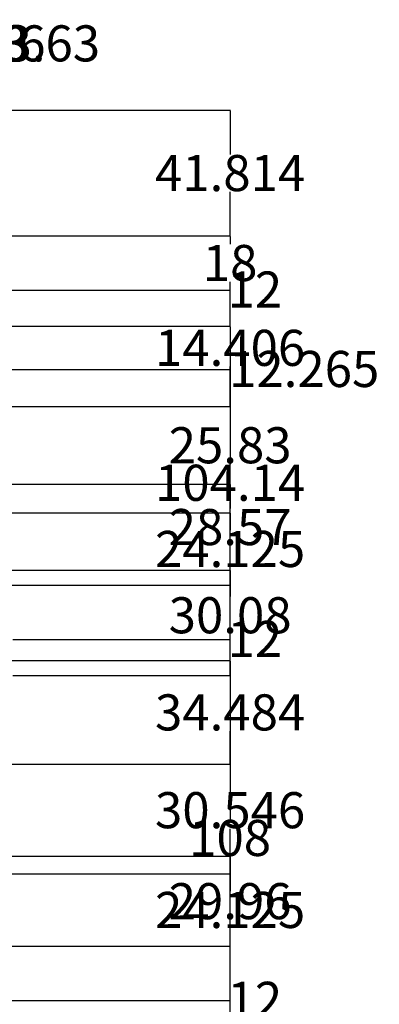
# Model space of a CAD drawing. Units: inches. Extents: x -73 to 458, y -161 to 332.
# Tile 6 of 6: x 338 to 458, y 5 to 332. Entities that reach past the tile are written whole.
import ezdxf

# ---------------------------------------------------------------- set-up
doc = ezdxf.new("R2010")
doc.units = ezdxf.units.IN
doc.header["$MEASUREMENT"] = 0
doc.layers.add('A-ANNO-DIMS', color=2, linetype='Continuous', lineweight=18)
doc.styles.get("Standard").update_dxf_attribs({"font": 'arial.ttf'})
doc.dimstyles.get("Standard").update_dxf_attribs({"dimtxt": 12, "dimasz": 0.18, "dimexe": 0.18, "dimexo": 0.0625, "dimgap": 0.09, "dimtad": 0, "dimtih": 1, "dimtoh": 1, "dimdec": 0, "dimzin": 0, "dimdsep": 46, "dimlunit": 3, "dimtxsty": 'Standard', "dimcen": 0.09, "dimadec": 0, "dimazin": 0, "dimtfac": 1, "dimtdec": 0, "dimtofl": 0, "dimtmove": 0, "dimatfit": 3, "dimfxl": 1, "dimtolj": 1, "dimtzin": 0, "dimarcsym": 0})

# ---------------------------------------------------------------- blocks, each defined once
blk = doc.blocks.new('*D18')
at = {"layer": 'A-ANNO-DIMS', "color": 0, "lineweight": -2, "transparency": 16777216}
for p, q in [((336.06, 6.07), (408.51, 6.07)), ((408.33, 6.07), (408.33, 6.25)), ((408.33, 6.25), (408.51, 6.25)), ((408.33, -5.75), (408.33, 5.89)), ((336.06, -5.93), (408.51, -5.93))]:
    blk.add_line(p, q, dxfattribs=at)
at = {"layer": 'A-ANNO-DIMS', "color": 0, "transparency": 16777216}
for points in [[(408.3, 5.89), (408.36, 5.89), (408.33, 6.07)], [(408.3, -5.75), (408.36, -5.75), (408.33, -5.93)]]:
    blk.add_solid(points, dxfattribs=at)
at = {"layer": 'Defpoints', "color": 0, "transparency": 16777216}
for p in [(336, 6.07), (408.33, 6.07), (336, -5.93)]:
    blk.add_point(p, dxfattribs=at)
at = {"layer": 'A-ANNO-DIMS', "color": 0, "transparency": 16777216, "insert": (416.56, 6.25), "char_height": 12, "attachment_point": 5}
blk.add_mtext('\\A1;12', dxfattribs=at)
blk = doc.blocks.new('*D20')
at = {"layer": 'A-ANNO-DIMS', "color": 0, "lineweight": -2, "transparency": 16777216}
for p, q in [((336.06, 114.07), (408.51, 114.07)), ((408.33, 113.89), (408.33, 66.28)), ((408.33, 6.25), (408.33, 53.85)), ((324.06, 6.07), (408.51, 6.07))]:
    blk.add_line(p, q, dxfattribs=at)
at = {"layer": 'A-ANNO-DIMS', "color": 0, "transparency": 16777216}
for points in [[(408.3, 113.89), (408.36, 113.89), (408.33, 114.07)], [(408.3, 6.25), (408.36, 6.25), (408.33, 6.07)]]:
    blk.add_solid(points, dxfattribs=at)
at = {"layer": 'Defpoints', "color": 0, "transparency": 16777216}
for p in [(336, 114.07), (408.33, 114.07), (324, 6.07)]:
    blk.add_point(p, dxfattribs=at)
at = {"layer": 'A-ANNO-DIMS', "color": 0, "transparency": 16777216, "insert": (408.33, 60.07), "char_height": 12, "attachment_point": 5}
blk.add_mtext('\\A1;108', dxfattribs=at)
blk = doc.blocks.new('*D21')
at = {"layer": 'A-ANNO-DIMS', "color": 0, "lineweight": -2, "transparency": 16777216}
for p, q in [((336.06, 126.07), (408.51, 126.07)), ((408.33, 126.07), (408.33, 126.25)), ((408.33, 126.25), (408.51, 126.25)), ((408.33, 114.25), (408.33, 125.89)), ((336.06, 114.07), (408.51, 114.07))]:
    blk.add_line(p, q, dxfattribs=at)
at = {"layer": 'A-ANNO-DIMS', "color": 0, "transparency": 16777216}
for points in [[(408.3, 125.89), (408.36, 125.89), (408.33, 126.07)], [(408.3, 114.25), (408.36, 114.25), (408.33, 114.07)]]:
    blk.add_solid(points, dxfattribs=at)
at = {"layer": 'Defpoints', "color": 0, "transparency": 16777216}
for p in [(336, 126.07), (408.33, 126.07), (336, 114.07)]:
    blk.add_point(p, dxfattribs=at)
at = {"layer": 'A-ANNO-DIMS', "color": 0, "transparency": 16777216, "insert": (416.56, 126.25), "char_height": 12, "attachment_point": 5}
blk.add_mtext('\\A1;12', dxfattribs=at)
blk = doc.blocks.new('*D22')
at = {"layer": 'A-ANNO-DIMS', "color": 0, "lineweight": -2, "transparency": 16777216}
for p, q in [((336.06, 230.21), (408.51, 230.21)), ((408.33, 230.03), (408.33, 184.35)), ((408.33, 126.25), (408.33, 171.92)), ((336.06, 126.07), (408.51, 126.07))]:
    blk.add_line(p, q, dxfattribs=at)
at = {"layer": 'A-ANNO-DIMS', "color": 0, "transparency": 16777216}
for points in [[(408.3, 230.03), (408.36, 230.03), (408.33, 230.21)], [(408.3, 126.25), (408.36, 126.25), (408.33, 126.07)]]:
    blk.add_solid(points, dxfattribs=at)
at = {"layer": 'Defpoints', "color": 0, "transparency": 16777216}
for p in [(336, 230.21), (408.33, 230.21), (336, 126.07)]:
    blk.add_point(p, dxfattribs=at)
at = {"layer": 'A-ANNO-DIMS', "color": 0, "transparency": 16777216, "insert": (408.33, 178.14), "char_height": 12, "attachment_point": 5}
blk.add_mtext('\\A1;104.14', dxfattribs=at)
blk = doc.blocks.new('*D23')
at = {"layer": 'A-ANNO-DIMS', "color": 0, "lineweight": -2, "transparency": 16777216}
for p, q in [((408.33, 242.21), (408.33, 242.39)), ((408.33, 242.39), (408.51, 242.39)), ((336.06, 242.21), (408.51, 242.21)), ((408.33, 230.39), (408.33, 242.03)), ((336.06, 230.21), (408.51, 230.21))]:
    blk.add_line(p, q, dxfattribs=at)
at = {"layer": 'A-ANNO-DIMS', "color": 0, "transparency": 16777216}
for points in [[(408.3, 242.03), (408.36, 242.03), (408.33, 242.21)], [(408.3, 230.39), (408.36, 230.39), (408.33, 230.21)]]:
    blk.add_solid(points, dxfattribs=at)
at = {"layer": 'Defpoints', "color": 0, "transparency": 16777216}
for p in [(336, 242.21), (408.33, 242.21), (336, 230.21)]:
    blk.add_point(p, dxfattribs=at)
at = {"layer": 'A-ANNO-DIMS', "color": 0, "transparency": 16777216, "insert": (416.56, 242.39), "char_height": 12, "attachment_point": 5}
blk.add_mtext('\\A1;12', dxfattribs=at)
blk = doc.blocks.new('*D24')
at = {"layer": 'A-ANNO-DIMS', "color": 0, "lineweight": -2, "transparency": 16777216}
for p, q in [((324.06, 260.21), (408.51, 260.21)), ((408.33, 260.03), (408.33, 257.42)), ((408.33, 242.39), (408.33, 244.99)), ((324.06, 242.21), (408.51, 242.21))]:
    blk.add_line(p, q, dxfattribs=at)
at = {"layer": 'A-ANNO-DIMS', "color": 0, "transparency": 16777216}
for points in [[(408.3, 260.03), (408.36, 260.03), (408.33, 260.21)], [(408.3, 242.39), (408.36, 242.39), (408.33, 242.21)]]:
    blk.add_solid(points, dxfattribs=at)
at = {"layer": 'Defpoints', "color": 0, "transparency": 16777216}
for p in [(324, 260.21), (408.33, 260.21), (324, 242.21)]:
    blk.add_point(p, dxfattribs=at)
at = {"layer": 'A-ANNO-DIMS', "color": 0, "transparency": 16777216, "insert": (408.33, 251.21), "char_height": 12, "attachment_point": 5}
blk.add_mtext('\\A1;18', dxfattribs=at)
blk = doc.blocks.new('*D25')
at = {"layer": 'A-ANNO-DIMS', "color": 0, "lineweight": -2, "transparency": 16777216}
for p, q in [((168.06, 302.02), (408.51, 302.02)), ((408.33, 301.84), (408.33, 287.33)), ((408.33, 260.39), (408.33, 274.9)), ((168.06, 260.21), (408.51, 260.21))]:
    blk.add_line(p, q, dxfattribs=at)
at = {"layer": 'A-ANNO-DIMS', "color": 0, "transparency": 16777216}
for points in [[(408.3, 301.84), (408.36, 301.84), (408.33, 302.02)], [(408.3, 260.39), (408.36, 260.39), (408.33, 260.21)]]:
    blk.add_solid(points, dxfattribs=at)
at = {"layer": 'Defpoints', "color": 0, "transparency": 16777216}
for p in [(168, 302.02), (408.33, 302.02), (168, 260.21)]:
    blk.add_point(p, dxfattribs=at)
at = {"layer": 'A-ANNO-DIMS', "color": 0, "transparency": 16777216, "insert": (408.33, 281.11), "char_height": 12, "attachment_point": 5}
blk.add_mtext('\\A1;41.814', dxfattribs=at)
blk = doc.blocks.new('*D39')
at = {"layer": 'A-ANNO-DIMS', "color": 0, "lineweight": -2, "transparency": 16777216}
for p, q in [((144.06, 54.03), (408.51, 54.03)), ((408.33, 53.85), (408.33, 45.26)), ((408.33, 24.25), (408.33, 32.83)), ((144.06, 24.07), (408.51, 24.07))]:
    blk.add_line(p, q, dxfattribs=at)
at = {"layer": 'A-ANNO-DIMS', "color": 0, "transparency": 16777216}
for points in [[(408.3, 53.85), (408.36, 53.85), (408.33, 54.03)], [(408.3, 24.25), (408.36, 24.25), (408.33, 24.07)]]:
    blk.add_solid(points, dxfattribs=at)
at = {"layer": 'Defpoints', "color": 0, "transparency": 16777216}
for p in [(144, 54.03), (408.33, 54.03), (144, 24.07)]:
    blk.add_point(p, dxfattribs=at)
at = {"layer": 'A-ANNO-DIMS', "color": 0, "transparency": 16777216, "insert": (408.33, 39.05), "char_height": 12, "attachment_point": 5}
blk.add_mtext('\\A1;29.96', dxfattribs=at)
blk = doc.blocks.new('*D40')
at = {"layer": 'A-ANNO-DIMS', "color": 0, "lineweight": -2, "transparency": 16777216}
for p, q in [((144.06, 84.57), (408.51, 84.57)), ((408.33, 84.39), (408.33, 75.52)), ((408.33, 54.21), (408.33, 63.08)), ((144.06, 54.03), (408.51, 54.03))]:
    blk.add_line(p, q, dxfattribs=at)
at = {"layer": 'A-ANNO-DIMS', "color": 0, "transparency": 16777216}
for points in [[(408.3, 84.39), (408.36, 84.39), (408.33, 84.57)], [(408.3, 54.21), (408.36, 54.21), (408.33, 54.03)]]:
    blk.add_solid(points, dxfattribs=at)
at = {"layer": 'Defpoints', "color": 0, "transparency": 16777216}
for p in [(144, 84.57), (408.33, 84.57), (144, 54.03)]:
    blk.add_point(p, dxfattribs=at)
at = {"layer": 'A-ANNO-DIMS', "color": 0, "transparency": 16777216, "insert": (408.33, 69.3), "char_height": 12, "attachment_point": 5}
blk.add_mtext('\\A1;30.546', dxfattribs=at)
blk = doc.blocks.new('*D41')
at = {"layer": 'A-ANNO-DIMS', "color": 0, "lineweight": -2, "transparency": 16777216}
for p, q in [((144.06, 119.06), (408.51, 119.06)), ((408.33, 118.88), (408.33, 108.04)), ((408.33, 84.75), (408.33, 95.59)), ((144.06, 84.57), (408.51, 84.57))]:
    blk.add_line(p, q, dxfattribs=at)
at = {"layer": 'A-ANNO-DIMS', "color": 0, "transparency": 16777216}
for points in [[(408.3, 118.88), (408.36, 118.88), (408.33, 119.06)], [(408.3, 84.75), (408.36, 84.75), (408.33, 84.57)]]:
    blk.add_solid(points, dxfattribs=at)
at = {"layer": 'Defpoints', "color": 0, "transparency": 16777216}
for p in [(144, 119.06), (408.33, 119.06), (144, 84.57)]:
    blk.add_point(p, dxfattribs=at)
at = {"layer": 'A-ANNO-DIMS', "color": 0, "transparency": 16777216, "insert": (408.33, 101.81), "char_height": 12, "attachment_point": 5}
blk.add_mtext('\\A1;34.484', dxfattribs=at)
blk = doc.blocks.new('*D42')
at = {"layer": 'A-ANNO-DIMS', "color": 0, "lineweight": -2, "transparency": 16777216}
for p, q in [((144.06, 149.14), (408.51, 149.14)), ((408.33, 148.96), (408.33, 140.32)), ((408.33, 119.24), (408.33, 127.88)), ((144.06, 119.06), (408.51, 119.06))]:
    blk.add_line(p, q, dxfattribs=at)
at = {"layer": 'A-ANNO-DIMS', "color": 0, "transparency": 16777216}
for points in [[(408.3, 148.96), (408.36, 148.96), (408.33, 149.14)], [(408.3, 119.24), (408.36, 119.24), (408.33, 119.06)]]:
    blk.add_solid(points, dxfattribs=at)
at = {"layer": 'Defpoints', "color": 0, "transparency": 16777216}
for p in [(144, 149.14), (408.33, 149.14), (144, 119.06)]:
    blk.add_point(p, dxfattribs=at)
at = {"layer": 'A-ANNO-DIMS', "color": 0, "transparency": 16777216, "insert": (408.33, 134.1), "char_height": 12, "attachment_point": 5}
blk.add_mtext('\\A1;30.08', dxfattribs=at)
blk = doc.blocks.new('*D43')
at = {"layer": 'A-ANNO-DIMS', "color": 0, "lineweight": -2, "transparency": 16777216}
for p, q in [((144.06, 177.7), (408.51, 177.7)), ((408.33, 177.52), (408.33, 169.64)), ((408.33, 149.32), (408.33, 157.2)), ((144.06, 149.14), (408.51, 149.14))]:
    blk.add_line(p, q, dxfattribs=at)
at = {"layer": 'A-ANNO-DIMS', "color": 0, "transparency": 16777216}
for points in [[(408.3, 177.52), (408.36, 177.52), (408.33, 177.7)], [(408.3, 149.32), (408.36, 149.32), (408.33, 149.14)]]:
    blk.add_solid(points, dxfattribs=at)
at = {"layer": 'Defpoints', "color": 0, "transparency": 16777216}
for p in [(144, 177.7), (408.33, 177.7), (144, 149.14)]:
    blk.add_point(p, dxfattribs=at)
at = {"layer": 'A-ANNO-DIMS', "color": 0, "transparency": 16777216, "insert": (408.33, 163.42), "char_height": 12, "attachment_point": 5}
blk.add_mtext('\\A1;28.57', dxfattribs=at)
blk = doc.blocks.new('*D44')
at = {"layer": 'A-ANNO-DIMS', "color": 0, "lineweight": -2, "transparency": 16777216}
for p, q in [((144.06, 203.54), (408.51, 203.54)), ((408.33, 203.36), (408.33, 196.84)), ((408.33, 177.88), (408.33, 184.4)), ((144.06, 177.7), (408.51, 177.7))]:
    blk.add_line(p, q, dxfattribs=at)
at = {"layer": 'A-ANNO-DIMS', "color": 0, "transparency": 16777216}
for points in [[(408.3, 203.36), (408.36, 203.36), (408.33, 203.54)], [(408.3, 177.88), (408.36, 177.88), (408.33, 177.7)]]:
    blk.add_solid(points, dxfattribs=at)
at = {"layer": 'Defpoints', "color": 0, "transparency": 16777216}
for p in [(144, 203.54), (408.33, 203.54), (144, 177.7)]:
    blk.add_point(p, dxfattribs=at)
at = {"layer": 'A-ANNO-DIMS', "color": 0, "transparency": 16777216, "insert": (408.33, 190.62), "char_height": 12, "attachment_point": 5}
blk.add_mtext('\\A1;25.83', dxfattribs=at)
blk = doc.blocks.new('*D45')
at = {"layer": 'A-ANNO-DIMS', "color": 0, "lineweight": -2, "transparency": 16777216}
for p, q in [((144.06, 215.8), (408.51, 215.8)), ((408.33, 215.8), (408.33, 215.98)), ((408.33, 215.98), (408.51, 215.98)), ((408.33, 203.72), (408.33, 215.62)), ((144.06, 203.54), (408.51, 203.54))]:
    blk.add_line(p, q, dxfattribs=at)
at = {"layer": 'A-ANNO-DIMS', "color": 0, "transparency": 16777216}
for points in [[(408.3, 215.62), (408.36, 215.62), (408.33, 215.8)], [(408.3, 203.72), (408.36, 203.72), (408.33, 203.54)]]:
    blk.add_solid(points, dxfattribs=at)
at = {"layer": 'Defpoints', "color": 0, "transparency": 16777216}
for p in [(144, 215.8), (408.33, 215.8), (144, 203.54)]:
    blk.add_point(p, dxfattribs=at)
at = {"layer": 'A-ANNO-DIMS', "color": 0, "transparency": 16777216, "insert": (432.98, 215.98), "char_height": 12, "attachment_point": 5}
blk.add_mtext('\\A1;12.265', dxfattribs=at)
blk = doc.blocks.new('*D46')
at = {"layer": 'A-ANNO-DIMS', "color": 0, "lineweight": -2, "transparency": 16777216}
for p, q in [((156.06, 230.21), (408.51, 230.21)), ((408.33, 230.03), (408.33, 229.22)), ((408.33, 215.98), (408.33, 216.79)), ((144.06, 215.8), (408.51, 215.8))]:
    blk.add_line(p, q, dxfattribs=at)
at = {"layer": 'A-ANNO-DIMS', "color": 0, "transparency": 16777216}
for points in [[(408.3, 230.03), (408.36, 230.03), (408.33, 230.21)], [(408.3, 215.98), (408.36, 215.98), (408.33, 215.8)]]:
    blk.add_solid(points, dxfattribs=at)
at = {"layer": 'Defpoints', "color": 0, "transparency": 16777216}
for p in [(156, 230.21), (408.33, 230.21), (144, 215.8)]:
    blk.add_point(p, dxfattribs=at)
at = {"layer": 'A-ANNO-DIMS', "color": 0, "transparency": 16777216, "insert": (408.33, 223), "char_height": 12, "attachment_point": 5}
blk.add_mtext('\\A1;14.406', dxfattribs=at)
blk = doc.blocks.new('*D58')
at = {"layer": 'A-ANNO-DIMS', "color": 0, "lineweight": -2, "transparency": 16777216}
for p, q in [((282.11, 168.25), (282.11, 324.4)), ((282.29, 324.22), (297.14, 324.22)), ((297.32, 168.25), (297.32, 324.4)), ((297.32, 324.22), (297.5, 324.22))]:
    blk.add_line(p, q, dxfattribs=at)
at = {"layer": 'A-ANNO-DIMS', "color": 0, "transparency": 16777216}
for points in [[(282.29, 324.25), (282.29, 324.19), (282.11, 324.22)], [(297.14, 324.25), (297.14, 324.19), (297.32, 324.22)]]:
    blk.add_solid(points, dxfattribs=at)
at = {"layer": 'Defpoints', "color": 0, "transparency": 16777216}
for p in [(297.32, 324.22), (282.11, 168.19), (297.32, 168.19)]:
    blk.add_point(p, dxfattribs=at)
at = {"layer": 'A-ANNO-DIMS', "color": 0, "transparency": 16777216, "insert": (321.93, 324.22), "char_height": 12, "attachment_point": 5}
blk.add_mtext('\\A1;15.216', dxfattribs=at)
blk = doc.blocks.new('*D59')
at = {"layer": 'A-ANNO-DIMS', "color": 0, "lineweight": -2, "transparency": 16777216}
for p, q in [((297.32, 168.25), (297.32, 324.4)), ((297.5, 324.22), (300.19, 324.22)), ((300.37, 168.25), (300.37, 324.4)), ((300.37, 324.22), (300.55, 324.22))]:
    blk.add_line(p, q, dxfattribs=at)
at = {"layer": 'A-ANNO-DIMS', "color": 0, "transparency": 16777216}
for points in [[(297.5, 324.25), (297.5, 324.19), (297.32, 324.22)], [(300.19, 324.25), (300.19, 324.19), (300.37, 324.22)]]:
    blk.add_solid(points, dxfattribs=at)
at = {"layer": 'Defpoints', "color": 0, "transparency": 16777216}
for p in [(300.37, 324.22), (297.32, 168.19), (300.37, 168.19)]:
    blk.add_point(p, dxfattribs=at)
at = {"layer": 'A-ANNO-DIMS', "color": 0, "transparency": 16777216, "insert": (320.88, 324.22), "char_height": 12, "attachment_point": 5}
blk.add_mtext('\\A1;3.043', dxfattribs=at)
blk = doc.blocks.new('*D60')
at = {"layer": 'A-ANNO-DIMS', "color": 0, "lineweight": -2, "transparency": 16777216}
for p, q in [((300.37, 168.25), (300.37, 324.4)), ((300.55, 324.22), (323.82, 324.22)), ((324, 168.25), (324, 324.4)), ((324, 324.22), (324.18, 324.22))]:
    blk.add_line(p, q, dxfattribs=at)
at = {"layer": 'A-ANNO-DIMS', "color": 0, "transparency": 16777216}
for points in [[(300.55, 324.25), (300.55, 324.19), (300.37, 324.22)], [(323.82, 324.25), (323.82, 324.19), (324, 324.22)]]:
    blk.add_solid(points, dxfattribs=at)
at = {"layer": 'Defpoints', "color": 0, "transparency": 16777216}
for p in [(324, 324.22), (300.37, 168.19), (324, 168.19)]:
    blk.add_point(p, dxfattribs=at)
at = {"layer": 'A-ANNO-DIMS', "color": 0, "transparency": 16777216, "insert": (344.62, 324.22), "char_height": 12, "attachment_point": 5}
blk.add_mtext('\\A1;23.63', dxfattribs=at)
blk = doc.blocks.new('*D69')
at = {"layer": 'A-ANNO-DIMS', "color": 0, "lineweight": -2, "transparency": 16777216}
for p, q in [((324.06, 168.19), (408.51, 168.19)), ((408.33, 168.01), (408.33, 162.35)), ((408.33, 144.25), (408.33, 149.91)), ((324.06, 144.07), (408.51, 144.07))]:
    blk.add_line(p, q, dxfattribs=at)
at = {"layer": 'A-ANNO-DIMS', "color": 0, "transparency": 16777216}
for points in [[(408.3, 168.01), (408.36, 168.01), (408.33, 168.19)], [(408.3, 144.25), (408.36, 144.25), (408.33, 144.07)]]:
    blk.add_solid(points, dxfattribs=at)
at = {"layer": 'Defpoints', "color": 0, "transparency": 16777216}
for p in [(324, 168.19), (408.33, 168.19), (324, 144.07)]:
    blk.add_point(p, dxfattribs=at)
at = {"layer": 'A-ANNO-DIMS', "color": 0, "transparency": 16777216, "insert": (408.33, 156.13), "char_height": 12, "attachment_point": 5}
blk.add_mtext('\\A1;24.125', dxfattribs=at)
blk = doc.blocks.new('*D70')
at = {"layer": 'A-ANNO-DIMS', "color": 0, "lineweight": -2, "transparency": 16777216}
for p, q in [((324.06, 48.19), (408.51, 48.19)), ((408.33, 48.01), (408.33, 42.35)), ((408.33, 24.25), (408.33, 29.91)), ((324.06, 24.07), (408.51, 24.07))]:
    blk.add_line(p, q, dxfattribs=at)
at = {"layer": 'A-ANNO-DIMS', "color": 0, "transparency": 16777216}
for points in [[(408.3, 48.01), (408.36, 48.01), (408.33, 48.19)], [(408.3, 24.25), (408.36, 24.25), (408.33, 24.07)]]:
    blk.add_solid(points, dxfattribs=at)
at = {"layer": 'Defpoints', "color": 0, "transparency": 16777216}
for p in [(324, 48.19), (408.33, 48.19), (324, 24.07)]:
    blk.add_point(p, dxfattribs=at)
at = {"layer": 'A-ANNO-DIMS', "color": 0, "transparency": 16777216, "insert": (408.33, 36.13), "char_height": 12, "attachment_point": 5}
blk.add_mtext('\\A1;24.125', dxfattribs=at)

msp = doc.modelspace()

# ---------------------------------------------------------------- dimensions: what is measured, and where the dimension line sits
at = {"layer": 'A-ANNO-DIMS'}
for base, p1, p2, override, picture, middle in [((297.3226, 324.2202), (282.107, 168.1912), (297.3226, 168.1912), {"dimdec": 3, "dimlfac": 1, "dimrnd": 0, "dimzin": 0, "dimdsep": 46, "dimlunit": 2}, '*D58', (321.9323, 324.2202)), ((300.3657, 324.2202), (297.3226, 168.1912), (300.3657, 168.1912), {"dimdec": 3, "dimlfac": 1, "dimrnd": 0, "dimzin": 0, "dimdsep": 46, "dimlunit": 2}, '*D59', (320.8786, 324.2202)), ((323.9979, 324.2202), (300.3657, 168.1912), (323.9979, 168.1912), {"dimdec": 2, "dimlfac": 1, "dimrnd": 0, "dimzin": 0, "dimdsep": 46, "dimlunit": 2}, '*D60', (344.6171, 324.2202))]:
    dim = msp.add_linear_dim(base=base, p1=p1, p2=p2, dimstyle='Standard', override=override, dxfattribs=at)
    dim.commit()
    dim.dimension.update_dxf_attribs({"geometry": picture, "text_midpoint": middle})
for base, p1, p2, override, picture, middle in [((408.326, 302.0202), (167.9979, 260.2059), (167.9979, 302.0202), {"dimdec": 3, "dimlfac": 1, "dimrnd": 0, "dimzin": 0, "dimdsep": 46, "dimlunit": 2}, '*D25', (408.326, 281.1131)), ((408.326, 260.2059), (323.9979, 242.2059), (323.9979, 260.2059), {"dimdec": 0, "dimlfac": 1, "dimrnd": 0, "dimzin": 0, "dimdsep": 46, "dimlunit": 2}, '*D24', (408.326, 251.2059)), ((408.326, 242.2059), (335.9979, 230.2059), (335.9979, 242.2059), {"dimdec": 0, "dimlfac": 1, "dimrnd": 0, "dimzin": 0, "dimdsep": 46, "dimlunit": 2}, '*D23', (416.5646, 242.3859)), ((408.326, 230.2059), (143.9979, 215.8003), (155.9979, 230.2059), {"dimdec": 3, "dimlfac": 1, "dimrnd": 0, "dimzin": 0, "dimdsep": 46, "dimlunit": 2}, '*D46', (408.326, 223.0031)), ((408.326, 230.2059), (335.9979, 126.0665), (335.9979, 230.2059), {"dimdec": 2, "dimlfac": 1, "dimrnd": 0, "dimzin": 0, "dimdsep": 46, "dimlunit": 2}, '*D22', (408.326, 178.1362)), ((408.326, 215.8003), (143.9979, 203.5354), (143.9979, 215.8003), {"dimdec": 3, "dimlfac": 1, "dimrnd": 0, "dimzin": 0, "dimdsep": 46, "dimlunit": 2}, '*D45', (432.9848, 215.9803)), ((408.326, 203.5354), (143.9979, 177.7045), (143.9979, 203.5354), {"dimdec": 2, "dimlfac": 1, "dimrnd": 0, "dimzin": 0, "dimdsep": 46, "dimlunit": 2}, '*D44', (408.326, 190.6199)), ((408.326, 177.7045), (143.9979, 149.136), (143.9979, 177.7045), {"dimdec": 2, "dimlfac": 1, "dimrnd": 0, "dimzin": 0, "dimdsep": 46, "dimlunit": 2}, '*D43', (408.326, 163.4203)), ((408.326, 168.1912), (323.9979, 144.0665), (323.9979, 168.1912), {"dimdec": 3, "dimlfac": 1, "dimrnd": 0, "dimzin": 0, "dimdsep": 46, "dimlunit": 2}, '*D69', (408.326, 156.1288)), ((408.326, 149.136), (143.9979, 119.0564), (143.9979, 149.136), {"dimdec": 2, "dimlfac": 1, "dimrnd": 0, "dimzin": 0, "dimdsep": 46, "dimlunit": 2}, '*D42', (408.326, 134.0962)), ((408.326, 126.0665), (335.9979, 114.0665), (335.9979, 126.0665), {"dimdec": 0, "dimlfac": 1, "dimrnd": 0, "dimzin": 0, "dimdsep": 46, "dimlunit": 2}, '*D21', (416.5646, 126.2465)), ((408.326, 119.0564), (143.9979, 84.5727), (143.9979, 119.0564), {"dimdec": 3, "dimlfac": 1, "dimrnd": 0, "dimzin": 0, "dimdsep": 46, "dimlunit": 2}, '*D41', (408.326, 101.8146)), ((408.326, 114.0665), (323.9979, 6.0665), (335.9979, 114.0665), {"dimdec": 0, "dimlfac": 1, "dimrnd": 0, "dimzin": 0, "dimdsep": 46, "dimlunit": 2}, '*D20', (408.326, 60.0665)), ((408.326, 84.5727), (143.9979, 54.0267), (143.9979, 84.5727), {"dimdec": 3, "dimlfac": 1, "dimrnd": 0, "dimzin": 0, "dimdsep": 46, "dimlunit": 2}, '*D40', (408.326, 69.2997)), ((408.326, 54.0267), (143.9979, 24.0665), (143.9979, 54.0267), {"dimdec": 2, "dimlfac": 1, "dimrnd": 0, "dimzin": 0, "dimdsep": 46, "dimlunit": 2}, '*D39', (408.326, 39.0466)), ((408.326, 48.1912), (323.9979, 24.0665), (323.9979, 48.1912), {"dimdec": 3, "dimlfac": 1, "dimrnd": 0, "dimzin": 0, "dimdsep": 46, "dimlunit": 2}, '*D70', (408.326, 36.1288)), ((408.326, 6.0665), (335.9979, -5.9335), (335.9979, 6.0665), {"dimdec": 0, "dimlfac": 1, "dimrnd": 0, "dimzin": 0, "dimdsep": 46, "dimlunit": 2}, '*D18', (416.5646, 6.2465))]:
    dim = msp.add_linear_dim(base=base, p1=p1, p2=p2, angle=90, dimstyle='Standard', override=override, dxfattribs=at)
    dim.commit()
    dim.dimension.update_dxf_attribs({"geometry": picture, "text_midpoint": middle})

doc.saveas('drawing.dxf')
